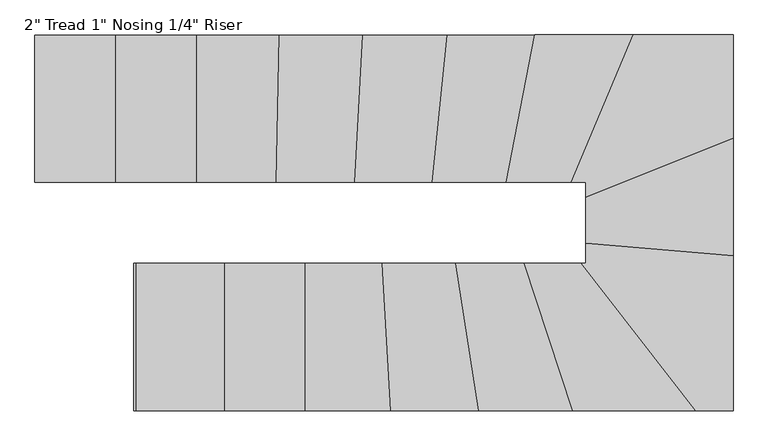
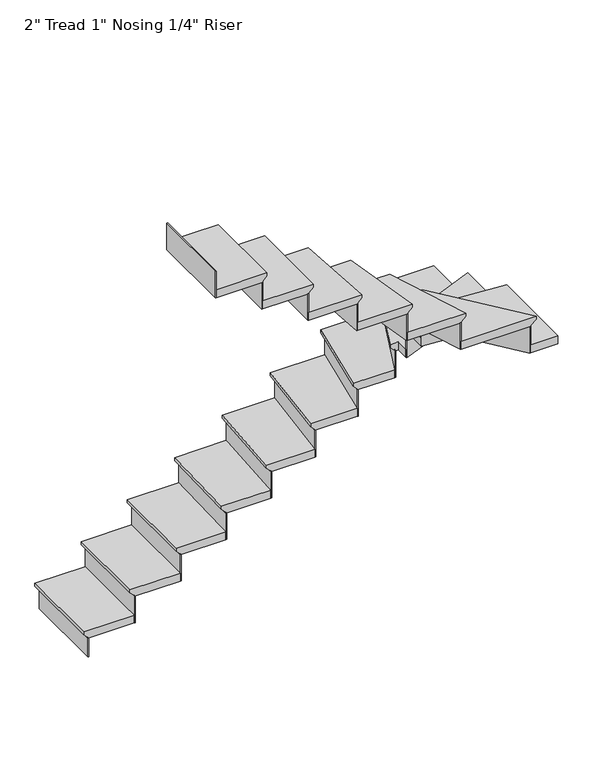
"""IFC4 building model written with IfcOpenShell, lengths in millimetres: stair flight geometry."""

from ifc_helpers import new_model, si_unit, origin, place, context, project, spatial, faceted_brep, source, transform, mapped, element, save


def stair_flight_42adf773(model_context):
    return source(origin(), model_context, "Body", "Brep", [
        faceted_brep([(838.4202681, 2693.877558, 319.6166667), (838.4202681, 2693.877558, 338.6666667), (838.4202681, 3202.4524989, 338.6666667), (838.4202681, 3202.4524989, 319.6166667), (863.8202681, 2693.877558, 294.2166667), (863.8202681, 3202.4524989, 294.2166667), (1143.2202681, 2693.877558, 338.6666667), (1143.2202681, 3202.4524989, 338.6666667), (863.8202681, 3202.4524989, 287.8666667), (1143.2202681, 3202.4524989, 287.8666667), (1143.2202681, 2693.877558, 287.8666667), (863.8202681, 2693.877558, 287.8666667)], [[[0, 1, 2, 3]], [[4, 0, 3, 5]], [[2, 1, 6, 7]], [[8, 9, 10, 11]], [[2, 7, 9, 8, 5, 3]], [[8, 11, 4, 5]], [[6, 1, 0, 4, 11, 10]], [[7, 6, 10, 9]]]),
        faceted_brep([(863.8202681, 2693.877558, 287.8666667), (863.8202681, 2693.877558, 169.3333333), (870.1702681, 2693.877558, 169.3333333), (870.1702681, 2693.877558, 287.8666667), (863.8202681, 3202.4524989, 287.8666667), (870.1702681, 3202.4524989, 287.8666667), (870.1702681, 3202.4524989, 169.3333333), (863.8202681, 3202.4524989, 169.3333333)], [[[0, 1, 2, 3]], [[4, 5, 6, 7]], [[1, 0, 4, 7]], [[2, 1, 7, 6]], [[3, 2, 6, 5]], [[0, 3, 5, 4]]]),
        faceted_brep([(1143.2202681, 2693.877558, 457.2), (1143.2202681, 2693.877558, 287.8666667), (1149.5702681, 2693.877558, 287.8666667), (1149.5702681, 2693.877558, 457.2), (1143.2202681, 3202.4524989, 457.2), (1149.5702681, 3202.4524989, 457.2), (1149.5702681, 3202.4524989, 287.8666667), (1143.2202681, 3202.4524989, 287.8666667)], [[[0, 1, 2, 3]], [[4, 5, 6, 7]], [[1, 0, 4, 7]], [[2, 1, 7, 6]], [[3, 2, 6, 5]], [[0, 3, 5, 4]]]),
        faceted_brep([(1117.8202681, 3202.4524989, 508.0), (1117.8202681, 2693.877558, 508.0), (1422.6202681, 2693.877558, 508.0), (1422.6202681, 3202.4524989, 508.0), (1143.2202681, 3202.4524989, 457.2), (1422.6202681, 3202.4524989, 457.2), (1422.6202681, 2693.877558, 457.2), (1143.2202681, 2693.877558, 457.2), (1143.2202681, 3202.4524989, 463.55), (1117.8202681, 3202.4524989, 488.95), (1143.2202681, 2693.877558, 463.55), (1117.8202681, 2693.877558, 488.95)], [[[0, 1, 2, 3]], [[4, 5, 6, 7]], [[0, 3, 5, 4, 8, 9]], [[4, 7, 10, 8]], [[2, 1, 11, 10, 7, 6]], [[3, 2, 6, 5]], [[11, 1, 0, 9]], [[10, 11, 9, 8]]]),
        faceted_brep([(1422.6202681, 2693.877558, 626.5333333), (1422.6202681, 2693.877558, 457.2), (1428.9702681, 2693.877558, 457.2), (1428.9702681, 2693.877558, 626.5333333), (1422.6202681, 3202.4524989, 626.5333333), (1428.9702681, 3202.4524989, 626.5333333), (1428.9702681, 3202.4524989, 457.2), (1422.6202681, 3202.4524989, 457.2)], [[[0, 1, 2, 3]], [[4, 5, 6, 7]], [[1, 0, 4, 7]], [[2, 1, 7, 6]], [[3, 2, 6, 5]], [[0, 3, 5, 4]]]),
        faceted_brep([(1397.2202681, 3202.4524989, 677.3333333), (1397.2202681, 2693.877558, 677.3333333), (1696.6553711, 2693.877558, 677.3333333), (1707.3964935, 3202.4524989, 677.3333333), (1422.6202681, 3202.4524989, 626.5333333), (1707.3964935, 3202.4524989, 626.5333333), (1696.6553711, 2693.877558, 626.5333333), (1422.6202681, 2693.877558, 626.5333333), (1422.6202681, 3202.4524989, 632.8833333), (1397.2202681, 3202.4524989, 658.2833333), (1422.6202681, 2693.877558, 632.8833333), (1397.2202681, 2693.877558, 658.2833333)], [[[0, 1, 2, 3]], [[4, 5, 6, 7]], [[0, 3, 5, 4, 8, 9]], [[4, 7, 10, 8]], [[2, 1, 11, 10, 7, 6]], [[3, 2, 6, 5]], [[11, 1, 0, 9]], [[10, 11, 9, 8]]]),
        faceted_brep([(1696.6553711, 2693.877558, 795.8666667), (1696.6553711, 2693.877558, 626.5333333), (1703.0067872, 2693.877558, 626.5333333), (1703.0067872, 2693.877558, 795.8666667), (1707.3964935, 3202.4524989, 795.8666667), (1713.7479096, 3202.4524989, 795.8666667), (1713.7479096, 3202.4524989, 626.5333333), (1707.3964935, 3202.4524989, 626.5333333)], [[[0, 1, 2, 3]], [[4, 5, 6, 7]], [[1, 0, 4, 7]], [[2, 1, 7, 6]], [[3, 2, 6, 5]], [[0, 3, 5, 4]]]),
        faceted_brep([(1681.9908293, 3202.4524989, 846.6666667), (1671.2497068, 2693.877558, 846.6666667), (1968.2389719, 2693.877558, 846.6666667), (1994.6701229, 3202.4524989, 846.6666667), (1707.3964935, 3202.4524989, 795.8666667), (1994.6701229, 3202.4524989, 795.8666667), (1968.2389719, 2693.877558, 795.8666667), (1696.6553711, 2693.877558, 795.8666667), (1707.3964935, 3202.4524989, 802.2166667), (1681.9908293, 3202.4524989, 827.6166667), (1696.6553711, 2693.877558, 802.2166667), (1671.2497068, 2693.877558, 827.6166667)], [[[0, 1, 2, 3]], [[4, 5, 6, 7]], [[0, 3, 5, 4, 8, 9]], [[4, 7, 10, 8]], [[2, 1, 11, 10, 7, 6]], [[3, 2, 6, 5]], [[11, 1, 0, 9]], [[10, 11, 9, 8]]]),
        faceted_brep([(1968.2389719, 2693.877558, 965.2), (1968.2389719, 2693.877558, 795.8666667), (1974.5975418, 2693.877558, 795.8666667), (1974.5975418, 2693.877558, 965.2), (1994.6701229, 3202.4524989, 965.2), (2001.0286928, 3202.4524989, 965.2), (2001.0286928, 3202.4524989, 795.8666667), (1994.6701229, 3202.4524989, 795.8666667)], [[[0, 1, 2, 3]], [[4, 5, 6, 7]], [[1, 0, 4, 7]], [[2, 1, 7, 6]], [[3, 2, 6, 5]], [[0, 3, 5, 4]]]),
        faceted_brep([(1969.2358436, 3202.4524989, 1016.0), (1942.8046925, 2693.877558, 1016.0), (2235.1931673, 2693.877558, 1016.0), (2286.7073051, 3202.4524989, 1016.0), (1994.6701229, 3202.4524989, 965.2), (2286.7073051, 3202.4524989, 965.2), (2235.1931673, 2693.877558, 965.2), (1968.2389719, 2693.877558, 965.2), (1994.6701229, 3202.4524989, 971.55), (1969.2358436, 3202.4524989, 996.95), (1968.2389719, 2693.877558, 971.55), (1942.8046925, 2693.877558, 996.95)], [[[0, 1, 2, 3]], [[4, 5, 6, 7]], [[0, 3, 5, 4, 8, 9]], [[4, 7, 10, 8]], [[2, 1, 11, 10, 7, 6]], [[3, 2, 6, 5]], [[11, 1, 0, 9]], [[10, 11, 9, 8]]]),
        faceted_brep([(2235.1931673, 2693.877558, 1134.5333333), (2235.1931673, 2693.877558, 965.2), (2241.5756594, 2693.877558, 965.2), (2241.5756594, 2693.877558, 1134.5333333), (2286.7073051, 3202.4524989, 1134.5333333), (2293.0897971, 3202.4524989, 1134.5333333), (2293.0897971, 3202.4524989, 965.2), (2286.7073051, 3202.4524989, 965.2)], [[[0, 1, 2, 3]], [[4, 5, 6, 7]], [[1, 0, 4, 7]], [[2, 1, 7, 6]], [[3, 2, 6, 5]], [[0, 3, 5, 4]]]),
        faceted_brep([(2261.1773369, 3202.4524989, 1185.3333333), (2209.6631992, 2693.877558, 1185.3333333), (2491.6737127, 2693.877558, 1185.3333333), (2589.7018996, 3202.4524989, 1185.3333333), (2286.7073051, 3202.4524989, 1134.5333333), (2589.7018996, 3202.4524989, 1134.5333333), (2491.6737127, 2693.877558, 1134.5333333), (2235.1931673, 2693.877558, 1134.5333333), (2286.7073051, 3202.4524989, 1140.8833333), (2261.1773369, 3202.4524989, 1166.2833333), (2235.1931673, 2693.877558, 1140.8833333), (2209.6631992, 2693.877558, 1166.2833333)], [[[0, 1, 2, 3]], [[4, 5, 6, 7]], [[0, 3, 5, 4, 8, 9]], [[4, 7, 10, 8]], [[2, 1, 11, 10, 7, 6]], [[3, 2, 6, 5]], [[11, 1, 0, 9]], [[10, 11, 9, 8]]]),
        faceted_brep([(2491.6737127, 2693.877558, 1303.8666667), (2491.6737127, 2693.877558, 1134.5333333), (2498.1405972, 2693.877558, 1134.5333333), (2498.1405972, 2693.877558, 1303.8666667), (2589.7018996, 3202.4524989, 1303.8666667), (2596.1687841, 3202.4524989, 1303.8666667), (2596.1687841, 3202.4524989, 1134.5333333), (2589.7018996, 3202.4524989, 1134.5333333)], [[[0, 1, 2, 3]], [[4, 5, 6, 7]], [[1, 0, 4, 7]], [[2, 1, 7, 6]], [[3, 2, 6, 5]], [[0, 3, 5, 4]]]),
        faceted_brep([(2563.8343615, 3202.4524989, 1354.6666667), (2465.8061746, 2693.877558, 1354.6666667), (2717.082711, 2693.877558, 1354.6666667), (2931.3822032, 3202.4524989, 1354.6666667), (2589.7018996, 3202.4524989, 1303.8666667), (2931.3822032, 3202.4524989, 1303.8666667), (2717.082711, 2693.877558, 1303.8666667), (2491.6737127, 2693.877558, 1303.8666667), (2589.7018996, 3202.4524989, 1310.2166667), (2563.8343615, 3202.4524989, 1335.6166667), (2491.6737127, 2693.877558, 1310.2166667), (2465.8061746, 2693.877558, 1335.6166667)], [[[0, 1, 2, 3]], [[4, 5, 6, 7]], [[0, 3, 5, 4, 8, 9]], [[4, 7, 10, 8]], [[2, 1, 11, 10, 7, 6]], [[3, 2, 6, 5]], [[11, 1, 0, 9]], [[10, 11, 9, 8]]]),
        faceted_brep([(2717.082711, 2693.877558, 1473.2), (2717.082711, 2693.877558, 1303.8666667), (2723.973426, 2693.877558, 1303.8666667), (2723.973426, 2693.877558, 1473.2), (2931.3822032, 3202.4524989, 1473.2), (2938.2729181, 3202.4524989, 1473.2), (2938.2729181, 3202.4524989, 1303.8666667), (2931.3822032, 3202.4524989, 1303.8666667)], [[[0, 1, 2, 3]], [[4, 5, 6, 7]], [[1, 0, 4, 7]], [[2, 1, 7, 6]], [[3, 2, 6, 5]], [[0, 3, 5, 4]]]),
        faceted_brep([(3247.982332, 2818.4435318, 1524.0), (3247.982332, 3202.4524989, 1524.0), (2903.8193433, 3202.4524989, 1524.0), (2689.5198512, 2693.877558, 1524.0), (2739.4073911, 2693.877558, 1524.0), (2739.4073911, 2614.5975609, 1524.0), (3247.982332, 3202.4524989, 1473.2), (3247.982332, 2818.4435318, 1473.2), (2739.4073911, 2614.5975609, 1473.2), (2739.4073911, 2693.877558, 1473.2), (2717.082711, 2693.877558, 1473.2), (2931.3822032, 3202.4524989, 1473.2), (2717.082711, 2693.877558, 1479.55), (2931.3822032, 3202.4524989, 1479.55), (2689.5198512, 2693.877558, 1504.95), (2903.8193433, 3202.4524989, 1504.95)], [[[0, 1, 2, 3, 4, 5]], [[6, 7, 8, 9, 10, 11]], [[1, 0, 7, 6]], [[11, 10, 12, 13]], [[5, 4, 9, 8]], [[0, 5, 8, 7]], [[14, 3, 2, 15]], [[12, 14, 15, 13]], [[4, 3, 14, 12, 10, 9]], [[2, 1, 6, 11, 13, 15]]]),
        faceted_brep([(2739.4073911, 2614.5975609, 1642.5333333), (2739.4073911, 2614.5975609, 1473.2), (2739.4073911, 2607.7564709, 1473.2), (2739.4073911, 2607.7564709, 1642.5333333), (3247.982332, 2818.4435318, 1642.5333333), (3247.982332, 2811.6024418, 1642.5333333), (3247.982332, 2811.6024418, 1473.2), (3247.982332, 2818.4435318, 1473.2)], [[[0, 1, 2, 3]], [[4, 5, 6, 7]], [[1, 0, 4, 7]], [[2, 1, 7, 6]], [[3, 2, 6, 5]], [[0, 3, 5, 4]]]),
        faceted_brep([(3247.982332, 2845.807892, 1693.3333333), (2739.4073911, 2641.9619211, 1693.3333333), (2739.4073911, 2458.7583414, 1693.3333333), (3247.982332, 2415.6151582, 1693.3333333), (3247.982332, 2818.4435318, 1642.5333333), (3247.982332, 2415.6151582, 1642.5333333), (2739.4073911, 2458.7583414, 1642.5333333), (2739.4073911, 2614.5975609, 1642.5333333), (3247.982332, 2818.4435318, 1648.8833333), (3247.982332, 2845.807892, 1674.2833333), (2739.4073911, 2614.5975609, 1648.8833333), (2739.4073911, 2641.9619211, 1674.2833333)], [[[0, 1, 2, 3]], [[4, 5, 6, 7]], [[0, 3, 5, 4, 8, 9]], [[4, 7, 10, 8]], [[2, 1, 11, 10, 7, 6]], [[3, 2, 6, 5]], [[11, 1, 0, 9]], [[10, 11, 9, 8]]]),
        faceted_brep([(2739.4073911, 2458.7583414, 1811.8666667), (2739.4073911, 2458.7583414, 1642.5333333), (2739.4073911, 2452.3855338, 1642.5333333), (2739.4073911, 2452.3855338, 1811.8666667), (3247.982332, 2415.6151582, 1811.8666667), (3247.982332, 2409.2423506, 1811.8666667), (3247.982332, 2409.2423506, 1642.5333333), (3247.982332, 2415.6151582, 1642.5333333)], [[[0, 1, 2, 3]], [[4, 5, 6, 7]], [[1, 0, 4, 7]], [[2, 1, 7, 6]], [[3, 2, 6, 5]], [[0, 3, 5, 4]]]),
        faceted_brep([(3085.5772675, 1905.9026171, 1862.6666667), (3247.982332, 1905.9026171, 1862.6666667), (3247.982332, 2441.1063885, 1862.6666667), (2739.4073911, 2484.2495716, 1862.6666667), (2739.4073911, 2414.477558, 1862.6666667), (2689.4386829, 2414.477558, 1862.6666667), (3247.982332, 1905.9026171, 1811.8666667), (3085.5772675, 1905.9026171, 1811.8666667), (2689.4386829, 2414.477558, 1811.8666667), (2739.4073911, 2414.477558, 1811.8666667), (2739.4073911, 2458.7583414, 1811.8666667), (3247.982332, 2415.6151582, 1811.8666667), (2739.4073911, 2458.7583414, 1818.2166667), (3247.982332, 2415.6151582, 1818.2166667), (2739.4073911, 2484.2495716, 1843.6166667), (3247.982332, 2441.1063885, 1843.6166667)], [[[0, 1, 2, 3, 4, 5]], [[6, 7, 8, 9, 10, 11]], [[1, 0, 7, 6]], [[11, 10, 12, 13]], [[4, 3, 14, 12, 10, 9]], [[5, 4, 9, 8]], [[0, 5, 8, 7]], [[14, 3, 2, 15]], [[12, 14, 15, 13]], [[2, 1, 6, 11, 13, 15]]]),
        faceted_brep([(2689.4386829, 2414.477558, 1981.2), (2689.4386829, 2414.477558, 1811.8666667), (2681.3896615, 2414.477558, 1811.8666667), (2681.3896615, 2414.477558, 1981.2), (3085.5772675, 1905.9026171, 1981.2), (3077.5282461, 1905.9026171, 1981.2), (3077.5282461, 1905.9026171, 1811.8666667), (3085.5772675, 1905.9026171, 1811.8666667)], [[[0, 1, 2, 3]], [[4, 5, 6, 7]], [[1, 0, 4, 7]], [[2, 1, 7, 6]], [[3, 2, 6, 5]], [[0, 3, 5, 4]]]),
        faceted_brep([(3117.7733531, 1905.9026171, 2032.0), (2721.6347685, 2414.477558, 2032.0), (2498.169104, 2414.477558, 2032.0), (2665.6971357, 1905.9026171, 2032.0), (3085.5772675, 1905.9026171, 1981.2), (2665.6971357, 1905.9026171, 1981.2), (2498.169104, 2414.477558, 1981.2), (2689.4386829, 2414.477558, 1981.2), (3085.5772675, 1905.9026171, 1987.55), (3117.7733531, 1905.9026171, 2012.95), (2689.4386829, 2414.477558, 1987.55), (2721.6347685, 2414.477558, 2012.95)], [[[0, 1, 2, 3]], [[4, 5, 6, 7]], [[0, 3, 5, 4, 8, 9]], [[4, 7, 10, 8]], [[2, 1, 11, 10, 7, 6]], [[3, 2, 6, 5]], [[11, 1, 0, 9]], [[10, 11, 9, 8]]]),
        faceted_brep([(2498.169104, 2414.477558, 2150.5333333), (2498.169104, 2414.477558, 1981.2), (2491.4834592, 2414.477558, 1981.2), (2491.4834592, 2414.477558, 2150.5333333), (2665.6971357, 1905.9026171, 2150.5333333), (2659.0114908, 1905.9026171, 2150.5333333), (2659.0114908, 1905.9026171, 1981.2), (2665.6971357, 1905.9026171, 1981.2)], [[[0, 1, 2, 3]], [[4, 5, 6, 7]], [[1, 0, 4, 7]], [[2, 1, 7, 6]], [[3, 2, 6, 5]], [[0, 3, 5, 4]]]),
        faceted_brep([(2692.4397151, 1905.9026171, 2201.3333333), (2524.9116834, 2414.477558, 2201.3333333), (2264.2527614, 2414.477558, 2201.3333333), (2342.8948816, 1905.9026171, 2201.3333333), (2665.6971357, 1905.9026171, 2150.5333333), (2342.8948816, 1905.9026171, 2150.5333333), (2264.2527614, 2414.477558, 2150.5333333), (2498.169104, 2414.477558, 2150.5333333), (2665.6971357, 1905.9026171, 2156.8833333), (2692.4397151, 1905.9026171, 2182.2833333), (2498.169104, 2414.477558, 2156.8833333), (2524.9116834, 2414.477558, 2182.2833333)], [[[0, 1, 2, 3]], [[4, 5, 6, 7]], [[0, 3, 5, 4, 8, 9]], [[4, 7, 10, 8]], [[2, 1, 11, 10, 7, 6]], [[3, 2, 6, 5]], [[11, 1, 0, 9]], [[10, 11, 9, 8]]]),
        faceted_brep([(2264.2527614, 2414.477558, 2319.8666667), (2264.2527614, 2414.477558, 2150.5333333), (2257.827292, 2414.477558, 2150.5333333), (2257.827292, 2414.477558, 2319.8666667), (2342.8948816, 1905.9026171, 2319.8666667), (2336.4694122, 1905.9026171, 2319.8666667), (2336.4694122, 1905.9026171, 2150.5333333), (2342.8948816, 1905.9026171, 2150.5333333)], [[[0, 1, 2, 3]], [[4, 5, 6, 7]], [[1, 0, 4, 7]], [[2, 1, 7, 6]], [[3, 2, 6, 5]], [[0, 3, 5, 4]]]),
        faceted_brep([(2368.5967594, 1905.9026171, 2370.6666667), (2289.9546392, 2414.477558, 2370.6666667), (2009.2587296, 2414.477558, 2370.6666667), (2039.6023306, 1905.9026171, 2370.6666667), (2342.8948816, 1905.9026171, 2319.8666667), (2039.6023306, 1905.9026171, 2319.8666667), (2009.2587296, 2414.477558, 2319.8666667), (2264.2527614, 2414.477558, 2319.8666667), (2342.8948816, 1905.9026171, 2326.2166667), (2368.5967594, 1905.9026171, 2351.6166667), (2264.2527614, 2414.477558, 2326.2166667), (2289.9546392, 2414.477558, 2351.6166667)], [[[0, 1, 2, 3]], [[4, 5, 6, 7]], [[0, 3, 5, 4, 8, 9]], [[4, 7, 10, 8]], [[2, 1, 11, 10, 7, 6]], [[3, 2, 6, 5]], [[11, 1, 0, 9]], [[10, 11, 9, 8]]]),
        faceted_brep([(2009.2587296, 2414.477558, 2489.2), (2009.2587296, 2414.477558, 2319.8666667), (2002.8974373, 2414.477558, 2319.8666667), (2002.8974373, 2414.477558, 2489.2), (2039.6023306, 1905.9026171, 2489.2), (2033.2410383, 1905.9026171, 2489.2), (2033.2410383, 1905.9026171, 2319.8666667), (2039.6023306, 1905.9026171, 2319.8666667)], [[[0, 1, 2, 3]], [[4, 5, 6, 7]], [[1, 0, 4, 7]], [[2, 1, 7, 6]], [[3, 2, 6, 5]], [[0, 3, 5, 4]]]),
        faceted_brep([(2065.0474997, 1905.9026171, 2540.0), (2034.7038988, 2414.477558, 2540.0), (1745.0756993, 2414.477558, 2540.0), (1745.0756993, 1905.9026171, 2540.0), (2039.6023306, 1905.9026171, 2489.2), (1745.0756993, 1905.9026171, 2489.2), (1745.0756993, 2414.477558, 2489.2), (2009.2587296, 2414.477558, 2489.2), (2039.6023306, 1905.9026171, 2495.55), (2065.0474997, 1905.9026171, 2520.95), (2009.2587296, 2414.477558, 2495.55), (2034.7038988, 2414.477558, 2520.95)], [[[0, 1, 2, 3]], [[4, 5, 6, 7]], [[0, 3, 5, 4, 8, 9]], [[4, 7, 10, 8]], [[2, 1, 11, 10, 7, 6]], [[3, 2, 6, 5]], [[11, 1, 0, 9]], [[10, 11, 9, 8]]]),
        faceted_brep([(1745.0756993, 2414.477558, 2658.5333333), (1745.0756993, 2414.477558, 2489.2), (1738.7256993, 2414.477558, 2489.2), (1738.7256993, 2414.477558, 2658.5333333), (1745.0756993, 1905.9026171, 2658.5333333), (1738.7256993, 1905.9026171, 2658.5333333), (1738.7256993, 1905.9026171, 2489.2), (1745.0756993, 1905.9026171, 2489.2)], [[[0, 1, 2, 3]], [[4, 5, 6, 7]], [[1, 0, 4, 7]], [[2, 1, 7, 6]], [[3, 2, 6, 5]], [[0, 3, 5, 4]]]),
        faceted_brep([(1770.4756993, 1905.9026171, 2709.3333333), (1770.4756993, 2414.477558, 2709.3333333), (1465.6756993, 2414.477558, 2709.3333333), (1465.6756993, 1905.9026171, 2709.3333333), (1745.0756993, 1905.9026171, 2658.5333333), (1465.6756993, 1905.9026171, 2658.5333333), (1465.6756993, 2414.477558, 2658.5333333), (1745.0756993, 2414.477558, 2658.5333333), (1745.0756993, 1905.9026171, 2664.8833333), (1770.4756993, 1905.9026171, 2690.2833333), (1745.0756993, 2414.477558, 2664.8833333), (1770.4756993, 2414.477558, 2690.2833333)], [[[0, 1, 2, 3]], [[4, 5, 6, 7]], [[0, 3, 5, 4, 8, 9]], [[4, 7, 10, 8]], [[2, 1, 11, 10, 7, 6]], [[3, 2, 6, 5]], [[11, 1, 0, 9]], [[10, 11, 9, 8]]]),
        faceted_brep([(1465.6756993, 2414.477558, 2827.8666667), (1465.6756993, 2414.477558, 2658.5333333), (1459.3256993, 2414.477558, 2658.5333333), (1459.3256993, 2414.477558, 2827.8666667), (1465.6756993, 1905.9026171, 2827.8666667), (1459.3256993, 1905.9026171, 2827.8666667), (1459.3256993, 1905.9026171, 2658.5333333), (1465.6756993, 1905.9026171, 2658.5333333)], [[[0, 1, 2, 3]], [[4, 5, 6, 7]], [[1, 0, 4, 7]], [[2, 1, 7, 6]], [[3, 2, 6, 5]], [[0, 3, 5, 4]]]),
        faceted_brep([(1186.2756993, 2414.477558, 2997.2), (1186.2756993, 2414.477558, 2827.8666667), (1179.9256993, 2414.477558, 2827.8666667), (1179.9256993, 2414.477558, 2997.2), (1186.2756993, 1905.9026171, 2997.2), (1179.9256993, 1905.9026171, 2997.2), (1179.9256993, 1905.9026171, 2827.8666667), (1186.2756993, 1905.9026171, 2827.8666667)], [[[0, 1, 2, 3]], [[4, 5, 6, 7]], [[1, 0, 4, 7]], [[2, 1, 7, 6]], [[3, 2, 6, 5]], [[0, 3, 5, 4]]]),
        faceted_brep([(1491.0756993, 1905.9026171, 2878.6666667), (1491.0756993, 2414.477558, 2878.6666667), (1186.2756993, 2414.477558, 2878.6666667), (1186.2756993, 1905.9026171, 2878.6666667), (1465.6756993, 1905.9026171, 2827.8666667), (1186.2756993, 1905.9026171, 2827.8666667), (1186.2756993, 2414.477558, 2827.8666667), (1465.6756993, 2414.477558, 2827.8666667), (1465.6756993, 1905.9026171, 2834.2166667), (1491.0756993, 1905.9026171, 2859.6166667), (1465.6756993, 2414.477558, 2834.2166667), (1491.0756993, 2414.477558, 2859.6166667)], [[[0, 1, 2, 3]], [[4, 5, 6, 7]], [[0, 3, 5, 4, 8, 9]], [[4, 7, 10, 8]], [[2, 1, 11, 10, 7, 6]], [[3, 2, 6, 5]], [[11, 1, 0, 9]], [[10, 11, 9, 8]]]),
    ])


if __name__ == "__main__":
    model = new_model("IFC4")
    model_context = context("Model", 3, world=origin())
    ifc_project = project(units=[si_unit("LENGTHUNIT", "METRE", prefix="MILLI")], contexts=[model_context])
    site = spatial("IfcSite", under=ifc_project)
    building = spatial("IfcBuilding", under=site)
    placement = place(None, origin())
    stair_flight_shape = stair_flight_42adf773(model_context)
    element("IfcStairFlight", 1, ObjectType="2\" Tread 1\" Nosing 1/4\" Riser", at=placement, inside=building, context=model_context, shape_type="MappedRepresentation", body=[
        mapped(stair_flight_shape, transform((0.0, 0.0, 0.0), x_axis=(1.0, 0.0, 0.0), y_axis=(0.0, 1.0, 0.0), z_axis=(0.0, 0.0, 1.0))),
    ])
    save(model, "model.ifc")
